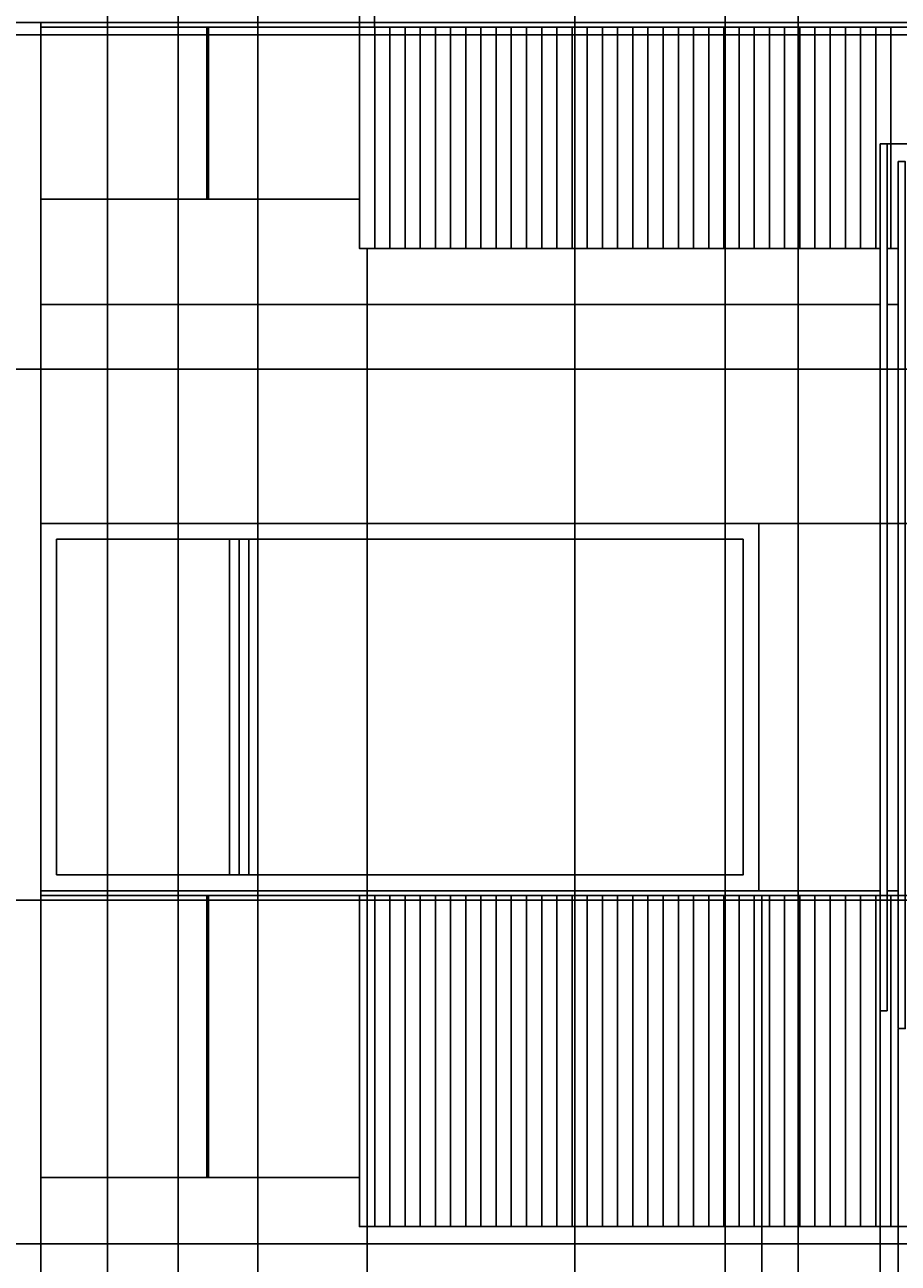
# Model space of a CAD drawing. Units: feet. Extents: x 2193 to 3502, y 890 to 1601.
# Tile 13 of 17: x 3145 to 3281, y 1076 to 1268. Entities that reach past the tile are written whole.
import ezdxf

# ---------------------------------------------------------------- set-up
doc = ezdxf.new("R2010")
doc.units = ezdxf.units.FT
doc.layers.add('A-ANNO-DIMS', color=2, linetype='Continuous', lineweight=18)
doc.layers.add('A-ELEV', color=7, linetype='Continuous', lineweight=25)
doc.styles.get("Standard").update_dxf_attribs({"font": 'arial.ttf'})
doc.dimstyles.get("Standard").update_dxf_attribs({"dimtxt": 0.18, "dimasz": 0.18, "dimexe": 0.18, "dimexo": 0.0625, "dimgap": 0.09, "dimtad": 0, "dimtih": 1, "dimtoh": 1, "dimdec": 0, "dimzin": 0, "dimdsep": 46, "dimlunit": 3, "dimtxsty": 'Standard', "dimcen": 0.09, "dimadec": 0, "dimazin": 0, "dimtfac": 1, "dimtdec": 0, "dimtofl": 0, "dimtmove": 0, "dimatfit": 3, "dimfxl": 1, "dimtolj": 1, "dimtzin": 0, "dimarcsym": 0})

# ---------------------------------------------------------------- blocks, each defined once
blk = doc.blocks.new('*D13')
at = {"layer": 'A-ANNO-DIMS', "color": 0, "lineweight": -2, "transparency": 16777216}
for p, q in [((2934.37, 950.89), (2934.37, 1601.47)), ((2934.55, 1601.29), (3186.64, 1601.29)), ((3439.51, 1601.29), (3187.43, 1601.29)), ((3439.69, 1541.11), (3439.69, 1601.47))]:
    blk.add_line(p, q, dxfattribs=at)
at = {"layer": 'A-ANNO-DIMS', "color": 0, "transparency": 16777216}
for points in [[(2934.55, 1601.32), (2934.55, 1601.26), (2934.37, 1601.29)], [(3439.51, 1601.32), (3439.51, 1601.26), (3439.69, 1601.29)]]:
    blk.add_solid(points, dxfattribs=at)
at = {"layer": 'Defpoints', "color": 0, "transparency": 16777216}
for p in [(3439.69, 1601.29), (3439.69, 1541.04), (2934.37, 950.82)]:
    blk.add_point(p, dxfattribs=at)
at = {"layer": 'A-ANNO-DIMS', "color": 0, "transparency": 16777216, "insert": (3187.03, 1601.29), "char_height": 0.18, "attachment_point": 5}
blk.add_mtext('\\A1;505.3', dxfattribs=at)
blk = doc.blocks.new('*D31')
at = {"layer": 'A-ANNO-DIMS', "color": 0, "lineweight": -2, "transparency": 16777216}
for p, q in [((2760.54, 1541.04), (3501.85, 1541.04)), ((3501.67, 1540.86), (3501.67, 1246.12)), ((3501.67, 951), (3501.67, 1245.75)), ((2762.27, 950.82), (3501.85, 950.82))]:
    blk.add_line(p, q, dxfattribs=at)
at = {"layer": 'A-ANNO-DIMS', "color": 0, "transparency": 16777216}
for points in [[(3501.64, 1540.86), (3501.7, 1540.86), (3501.67, 1541.04)], [(3501.64, 951), (3501.7, 951), (3501.67, 950.82)]]:
    blk.add_solid(points, dxfattribs=at)
at = {"layer": 'Defpoints', "color": 0, "transparency": 16777216}
for p in [(2760.47, 1541.04), (3501.67, 1541.04), (2762.2, 950.82)]:
    blk.add_point(p, dxfattribs=at)
at = {"layer": 'A-ANNO-DIMS', "color": 0, "transparency": 16777216, "insert": (3501.67, 1245.93), "char_height": 0.18, "attachment_point": 5}
blk.add_mtext('\\A1;590.2', dxfattribs=at)
blk = doc.blocks.new('*D61')
at = {"layer": 'A-ANNO-DIMS', "color": 0, "lineweight": -2, "transparency": 16777216}
for p, q in [((2974.12, 1078.97), (2974.12, 890.39)), ((3147.5, 1078.97), (3147.5, 890.39)), ((2974.3, 890.57), (3060.42, 890.57)), ((3147.32, 890.57), (3061.19, 890.57))]:
    blk.add_line(p, q, dxfattribs=at)
at = {"layer": 'A-ANNO-DIMS', "color": 0, "transparency": 16777216}
for points in [[(2974.3, 890.6), (2974.3, 890.54), (2974.12, 890.57)], [(3147.32, 890.6), (3147.32, 890.54), (3147.5, 890.57)]]:
    blk.add_solid(points, dxfattribs=at)
at = {"layer": 'Defpoints', "color": 0, "transparency": 16777216}
for p in [(2974.12, 1079.03), (3147.5, 1079.03), (3147.5, 890.57)]:
    blk.add_point(p, dxfattribs=at)
at = {"layer": 'A-ANNO-DIMS', "color": 0, "transparency": 16777216, "insert": (3060.81, 890.57), "char_height": 0.18, "attachment_point": 5}
blk.add_mtext('\\A1;173.4', dxfattribs=at)
blk = doc.blocks.new('*D62')
at = {"layer": 'A-ANNO-DIMS', "color": 0, "lineweight": -2, "transparency": 16777216}
for p, q in [((2974.18, 1266.71), (3501.85, 1266.71)), ((3501.67, 1266.53), (3501.67, 1173.05)), ((3501.67, 1079.21), (3501.67, 1172.69)), ((2974.18, 1079.03), (3501.85, 1079.03))]:
    blk.add_line(p, q, dxfattribs=at)
at = {"layer": 'A-ANNO-DIMS', "color": 0, "transparency": 16777216}
for points in [[(3501.64, 1266.53), (3501.7, 1266.53), (3501.67, 1266.71)], [(3501.64, 1079.21), (3501.7, 1079.21), (3501.67, 1079.03)]]:
    blk.add_solid(points, dxfattribs=at)
at = {"layer": 'Defpoints', "color": 0, "transparency": 16777216}
for p in [(2974.12, 1266.71), (3501.67, 1266.71), (2974.12, 1079.03)]:
    blk.add_point(p, dxfattribs=at)
at = {"layer": 'A-ANNO-DIMS', "color": 0, "transparency": 16777216, "insert": (3501.67, 1172.87), "char_height": 0.18, "attachment_point": 5}
blk.add_mtext('\\A1;187.68', dxfattribs=at)
blk = doc.blocks.new('*D67')
at = {"layer": 'A-ANNO-DIMS', "color": 0, "lineweight": -2, "transparency": 16777216}
for p, q in [((2980.78, 1214.84), (3501.85, 1214.84)), ((3501.67, 1214.66), (3501.67, 1173.8)), ((3501.67, 1132.57), (3501.67, 1173.43)), ((2980.78, 1132.39), (3501.85, 1132.39))]:
    blk.add_line(p, q, dxfattribs=at)
at = {"layer": 'A-ANNO-DIMS', "color": 0, "transparency": 16777216}
for points in [[(3501.64, 1214.66), (3501.7, 1214.66), (3501.67, 1214.84)], [(3501.64, 1132.57), (3501.7, 1132.57), (3501.67, 1132.39)]]:
    blk.add_solid(points, dxfattribs=at)
at = {"layer": 'Defpoints', "color": 0, "transparency": 16777216}
for p in [(2980.72, 1214.84), (3501.67, 1214.84), (2980.72, 1132.39)]:
    blk.add_point(p, dxfattribs=at)
at = {"layer": 'A-ANNO-DIMS', "color": 0, "transparency": 16777216, "insert": (3501.67, 1173.62), "char_height": 0.18, "attachment_point": 5}
blk.add_mtext('\\A1;82.44', dxfattribs=at)
blk = doc.blocks.new('*D76')
at = {"layer": 'A-ANNO-DIMS', "color": 0, "lineweight": -2, "transparency": 16777216}
for p, q in [((3259.05, 1190.87), (3501.85, 1190.87)), ((3501.67, 1190.69), (3501.67, 1162.17)), ((3501.67, 1133.29), (3501.67, 1161.81)), ((3259.52, 1133.11), (3501.85, 1133.11))]:
    blk.add_line(p, q, dxfattribs=at)
at = {"layer": 'A-ANNO-DIMS', "color": 0, "transparency": 16777216}
for points in [[(3501.64, 1190.69), (3501.7, 1190.69), (3501.67, 1190.87)], [(3501.64, 1133.29), (3501.7, 1133.29), (3501.67, 1133.11)]]:
    blk.add_solid(points, dxfattribs=at)
at = {"layer": 'Defpoints', "color": 0, "transparency": 16777216}
for p in [(3258.98, 1190.87), (3501.67, 1190.87), (3259.46, 1133.11)]:
    blk.add_point(p, dxfattribs=at)
at = {"layer": 'A-ANNO-DIMS', "color": 0, "transparency": 16777216, "insert": (3501.67, 1161.99), "char_height": 0.18, "attachment_point": 5}
blk.add_mtext('\\A1;57.75', dxfattribs=at)
blk = doc.blocks.new('*D80')
at = {"layer": 'A-ANNO-DIMS', "color": 0, "lineweight": -2, "transparency": 16777216}
for p, q in [((3198.15, 1233.5), (3198.15, 890.39)), ((3315.74, 1233.5), (3315.74, 890.39)), ((3198.33, 890.57), (3256.49, 890.57)), ((3315.56, 890.57), (3257.4, 890.57))]:
    blk.add_line(p, q, dxfattribs=at)
at = {"layer": 'A-ANNO-DIMS', "color": 0, "transparency": 16777216}
for points in [[(3198.33, 890.6), (3198.33, 890.54), (3198.15, 890.57)], [(3315.56, 890.6), (3315.56, 890.54), (3315.74, 890.57)]]:
    blk.add_solid(points, dxfattribs=at)
at = {"layer": 'Defpoints', "color": 0, "transparency": 16777216}
for p in [(3198.15, 1233.56), (3315.74, 1233.56), (3315.74, 890.57)]:
    blk.add_point(p, dxfattribs=at)
at = {"layer": 'A-ANNO-DIMS', "color": 0, "transparency": 16777216, "insert": (3256.94, 890.57), "char_height": 0.18, "attachment_point": 5}
blk.add_mtext('\\A1;117.58', dxfattribs=at)
blk = doc.blocks.new('*D83')
at = {"layer": 'A-ANNO-DIMS', "color": 0, "lineweight": -2, "transparency": 16777216}
for p, q in [((3147.5, 1133.05), (3147.5, 890.39)), ((3198.15, 1133.05), (3198.15, 890.39)), ((3147.68, 890.57), (3172.43, 890.57)), ((3197.97, 890.57), (3173.22, 890.57))]:
    blk.add_line(p, q, dxfattribs=at)
at = {"layer": 'A-ANNO-DIMS', "color": 0, "transparency": 16777216}
for points in [[(3147.68, 890.6), (3147.68, 890.54), (3147.5, 890.57)], [(3197.97, 890.6), (3197.97, 890.54), (3198.15, 890.57)]]:
    blk.add_solid(points, dxfattribs=at)
at = {"layer": 'Defpoints', "color": 0, "transparency": 16777216}
for p in [(3147.5, 1133.11), (3198.15, 1133.11), (3198.15, 890.57)]:
    blk.add_point(p, dxfattribs=at)
at = {"layer": 'A-ANNO-DIMS', "color": 0, "transparency": 16777216, "insert": (3172.83, 890.57), "char_height": 0.18, "attachment_point": 5}
blk.add_mtext('\\A1;50.65', dxfattribs=at)
blk = doc.blocks.new('*D84')
at = {"layer": 'A-ANNO-DIMS', "color": 0, "lineweight": -2, "transparency": 16777216}
for p, q in [((3196.98, 1267.98), (3196.98, 1601.47)), ((3197.16, 1601.29), (3197.76, 1601.29)), ((3199.15, 1601.29), (3198.55, 1601.29)), ((3199.33, 1267.98), (3199.33, 1601.47))]:
    blk.add_line(p, q, dxfattribs=at)
at = {"layer": 'A-ANNO-DIMS', "color": 0, "transparency": 16777216}
for points in [[(3197.16, 1601.32), (3197.16, 1601.26), (3196.98, 1601.29)], [(3199.15, 1601.32), (3199.15, 1601.26), (3199.33, 1601.29)]]:
    blk.add_solid(points, dxfattribs=at)
at = {"layer": 'Defpoints', "color": 0, "transparency": 16777216}
for p in [(3199.33, 1601.29), (3196.98, 1267.92), (3199.33, 1267.92)]:
    blk.add_point(p, dxfattribs=at)
at = {"layer": 'A-ANNO-DIMS', "color": 0, "transparency": 16777216, "insert": (3198.15, 1601.29), "char_height": 0.18, "attachment_point": 5}
blk.add_mtext('\\A1;2.358', dxfattribs=at)
blk = doc.blocks.new('*D85')
at = {"layer": 'A-ANNO-DIMS', "color": 0, "lineweight": -2, "transparency": 16777216}
for p, q in [((3259.46, 1133.05), (3259.46, 890.39)), ((3277.81, 1115.17), (3277.81, 890.39)), ((3259.64, 890.57), (3268.25, 890.57)), ((3277.63, 890.57), (3269.02, 890.57))]:
    blk.add_line(p, q, dxfattribs=at)
at = {"layer": 'A-ANNO-DIMS', "color": 0, "transparency": 16777216}
for points in [[(3259.64, 890.6), (3259.64, 890.54), (3259.46, 890.57)], [(3277.63, 890.6), (3277.63, 890.54), (3277.81, 890.57)]]:
    blk.add_solid(points, dxfattribs=at)
at = {"layer": 'Defpoints', "color": 0, "transparency": 16777216}
for p in [(3259.46, 1133.11), (3277.81, 1115.23), (3277.81, 890.57)]:
    blk.add_point(p, dxfattribs=at)
at = {"layer": 'A-ANNO-DIMS', "color": 0, "transparency": 16777216, "insert": (3268.63, 890.57), "char_height": 0.18, "attachment_point": 5}
blk.add_mtext('\\A1;18.35', dxfattribs=at)
blk = doc.blocks.new('*D86')
at = {"layer": 'A-ANNO-DIMS', "color": 0, "lineweight": -2, "transparency": 16777216}
for p, q in [((3277.81, 1115.17), (3277.81, 890.39)), ((3280.64, 1112.39), (3280.64, 890.39)), ((3277.99, 890.57), (3278.83, 890.57)), ((3280.46, 890.57), (3279.62, 890.57))]:
    blk.add_line(p, q, dxfattribs=at)
at = {"layer": 'A-ANNO-DIMS', "color": 0, "transparency": 16777216}
for points in [[(3277.99, 890.6), (3277.99, 890.54), (3277.81, 890.57)], [(3280.46, 890.6), (3280.46, 890.54), (3280.64, 890.57)]]:
    blk.add_solid(points, dxfattribs=at)
at = {"layer": 'Defpoints', "color": 0, "transparency": 16777216}
for p in [(3277.81, 1115.23), (3280.64, 1112.45), (3280.64, 890.57)]:
    blk.add_point(p, dxfattribs=at)
at = {"layer": 'A-ANNO-DIMS', "color": 0, "transparency": 16777216, "insert": (3279.22, 890.57), "char_height": 0.18, "attachment_point": 5}
blk.add_mtext('\\A1;2.832', dxfattribs=at)
blk = doc.blocks.new('*D91')
at = {"layer": 'A-ANNO-DIMS', "color": 0, "lineweight": -2, "transparency": 16777216}
for p, q in [((3277.2, 1267.92), (3501.85, 1267.92)), ((3501.67, 1267.74), (3501.67, 1259.05)), ((3501.67, 1250.01), (3501.67, 1258.69)), ((3277.87, 1249.83), (3501.85, 1249.83))]:
    blk.add_line(p, q, dxfattribs=at)
at = {"layer": 'A-ANNO-DIMS', "color": 0, "transparency": 16777216}
for points in [[(3501.64, 1267.74), (3501.7, 1267.74), (3501.67, 1267.92)], [(3501.64, 1250.01), (3501.7, 1250.01), (3501.67, 1249.83)]]:
    blk.add_solid(points, dxfattribs=at)
at = {"layer": 'Defpoints', "color": 0, "transparency": 16777216}
for p in [(3277.14, 1267.92), (3501.67, 1267.92), (3277.81, 1249.83)]:
    blk.add_point(p, dxfattribs=at)
at = {"layer": 'A-ANNO-DIMS', "color": 0, "transparency": 16777216, "insert": (3501.67, 1258.87), "char_height": 0.18, "attachment_point": 5}
blk.add_mtext('\\A1;18.09', dxfattribs=at)
blk = doc.blocks.new('*D97')
at = {"layer": 'A-ANNO-DIMS', "color": 0, "lineweight": -2, "transparency": 16777216}
for p, q in [((3111.13, 1032.26), (3111.13, 1601.47)), ((3111.31, 1601.29), (3207.6, 1601.29)), ((3304.79, 1601.29), (3208.51, 1601.29)), ((3304.97, 1032.26), (3304.97, 1601.47))]:
    blk.add_line(p, q, dxfattribs=at)
at = {"layer": 'A-ANNO-DIMS', "color": 0, "transparency": 16777216}
for points in [[(3111.31, 1601.32), (3111.31, 1601.26), (3111.13, 1601.29)], [(3304.79, 1601.32), (3304.79, 1601.26), (3304.97, 1601.29)]]:
    blk.add_solid(points, dxfattribs=at)
at = {"layer": 'Defpoints', "color": 0, "transparency": 16777216}
for p in [(3304.97, 1601.29), (3111.13, 1032.19), (3304.97, 1032.19)]:
    blk.add_point(p, dxfattribs=at)
at = {"layer": 'A-ANNO-DIMS', "color": 0, "transparency": 16777216, "insert": (3208.05, 1601.29), "char_height": 0.18, "attachment_point": 5}
blk.add_mtext('\\A1;193.84', dxfattribs=at)
blk = doc.blocks.new('*D100')
at = {"layer": 'A-ANNO-DIMS', "color": 0, "lineweight": -2, "transparency": 16777216}
for p, q in [((3168.83, 1055.37), (3168.83, 1601.47)), ((3169.01, 1601.29), (3216.57, 1601.29)), ((3264.92, 1601.29), (3217.36, 1601.29)), ((3265.1, 1055.37), (3265.1, 1601.47))]:
    blk.add_line(p, q, dxfattribs=at)
at = {"layer": 'A-ANNO-DIMS', "color": 0, "transparency": 16777216}
for points in [[(3169.01, 1601.32), (3169.01, 1601.26), (3168.83, 1601.29)], [(3264.92, 1601.32), (3264.92, 1601.26), (3265.1, 1601.29)]]:
    blk.add_solid(points, dxfattribs=at)
at = {"layer": 'Defpoints', "color": 0, "transparency": 16777216}
for p in [(3265.1, 1601.29), (3168.83, 1055.31), (3265.1, 1055.31)]:
    blk.add_point(p, dxfattribs=at)
at = {"layer": 'A-ANNO-DIMS', "color": 0, "transparency": 16777216, "insert": (3216.97, 1601.29), "char_height": 0.18, "attachment_point": 5}
blk.add_mtext('\\A1;96.27', dxfattribs=at)
blk = doc.blocks.new('*D104')
at = {"layer": 'A-ANNO-DIMS', "color": 0, "lineweight": -2, "transparency": 16777216}
for p, q in [((3157.83, 1001.2), (3157.83, 1601.47)), ((3158.01, 1601.29), (3169.1, 1601.29)), ((3180.99, 1601.29), (3169.89, 1601.29)), ((3181.17, 1001.2), (3181.17, 1601.47))]:
    blk.add_line(p, q, dxfattribs=at)
at = {"layer": 'A-ANNO-DIMS', "color": 0, "transparency": 16777216}
for points in [[(3158.01, 1601.32), (3158.01, 1601.26), (3157.83, 1601.29)], [(3180.99, 1601.32), (3180.99, 1601.26), (3181.17, 1601.29)]]:
    blk.add_solid(points, dxfattribs=at)
at = {"layer": 'Defpoints', "color": 0, "transparency": 16777216}
for p in [(3181.17, 1601.29), (3157.83, 1001.13), (3181.17, 1001.13)]:
    blk.add_point(p, dxfattribs=at)
at = {"layer": 'A-ANNO-DIMS', "color": 0, "transparency": 16777216, "insert": (3169.5, 1601.29), "char_height": 0.18, "attachment_point": 5}
blk.add_mtext('\\A1;23.34', dxfattribs=at)
blk = doc.blocks.new('*D106')
at = {"layer": 'A-ANNO-DIMS', "color": 0, "lineweight": -2, "transparency": 16777216}
for p, q in [((3230.44, 1001.2), (3230.44, 1601.47)), ((3230.62, 1601.29), (3241.72, 1601.29)), ((3253.6, 1601.29), (3242.51, 1601.29)), ((3253.78, 1001.2), (3253.78, 1601.47))]:
    blk.add_line(p, q, dxfattribs=at)
at = {"layer": 'A-ANNO-DIMS', "color": 0, "transparency": 16777216}
for points in [[(3230.62, 1601.32), (3230.62, 1601.26), (3230.44, 1601.29)], [(3253.6, 1601.32), (3253.6, 1601.26), (3253.78, 1601.29)]]:
    blk.add_solid(points, dxfattribs=at)
at = {"layer": 'Defpoints', "color": 0, "transparency": 16777216}
for p in [(3253.78, 1601.29), (3230.44, 1001.13), (3253.78, 1001.13)]:
    blk.add_point(p, dxfattribs=at)
at = {"layer": 'A-ANNO-DIMS', "color": 0, "transparency": 16777216, "insert": (3242.11, 1601.29), "char_height": 0.18, "attachment_point": 5}
blk.add_mtext('\\A1;23.34', dxfattribs=at)

msp = doc.modelspace()

# ---------------------------------------------------------------- linework, layer by layer
at = {"layer": 'A-ELEV'}
for p, q in [((3147.5022, 1241.1967), (3196.9758, 1241.1967)), ((3147.5022, 1224.865), (3277.8077, 1224.865)), ((3278.9051, 1224.865), (3280.6398, 1224.865)), ((3147.5022, 1089.3627), (3196.9758, 1089.3627))]:
    msp.add_line(p, q, dxfattribs=at)
for points in [[(2974.116, 1266.7092), (3147.5022, 1266.7092), (3147.5022, 1268.6599), (2974.116, 1268.6599)], [(2974.116, 1079.031), (3147.5022, 1079.031), (3147.5022, 1266.7092), (2974.116, 1266.7092)], [(3277.8077, 1249.8256), (3278.9051, 1249.8256), (3278.9051, 1115.2331), (3277.8077, 1115.2331)], [(3280.6398, 1247.0422), (3281.7371, 1247.0422), (3281.7371, 1112.4498), (3280.6398, 1112.4498)], [(3147.5022, 1133.8558), (3258.9838, 1133.8558), (3258.9838, 1190.8659), (3147.5022, 1190.8659)], [(3149.9473, 1136.3009), (3256.5386, 1136.3009), (3256.5386, 1188.4208), (3149.9473, 1188.4208)], [(3176.7885, 1188.4208), (3178.3021, 1188.4208), (3178.3021, 1136.3009), (3176.7885, 1136.3009)], [(3178.3021, 1188.4208), (3179.8157, 1188.4208), (3179.8157, 1136.3009), (3178.3021, 1136.3009)], [(3173.2631, 1133.1128), (3173.5128, 1133.1128), (3173.5128, 1089.3627), (3173.2631, 1089.3627)]]:
    msp.add_lwpolyline(points, close=True, dxfattribs=at)
for points in [[(3378.849, 1267.9169), (3147.5022, 1267.9169), (3147.5022, 1268.6599), (3378.849, 1268.6599)], [(3173.5128, 1267.9169), (3173.5128, 1241.1967), (3173.2631, 1241.1967), (3173.2631, 1267.9169)], [(3277.8077, 1233.561), (3196.9758, 1233.561), (3196.9758, 1267.9169)], [(3199.3336, 1267.9169), (3199.3336, 1233.561), (3198.1547, 1233.561)], [(3201.6915, 1267.9169), (3201.6915, 1233.561), (3200.5126, 1233.561)], [(3204.0493, 1267.9169), (3204.0493, 1233.561), (3202.8704, 1233.561)], [(3206.4072, 1267.9169), (3206.4072, 1233.561), (3205.2282, 1233.561)], [(3208.765, 1267.9169), (3208.765, 1233.561), (3207.5861, 1233.561)], [(3211.1228, 1267.9169), (3211.1228, 1233.561), (3209.9439, 1233.561)], [(3213.4807, 1267.9169), (3213.4807, 1233.561), (3212.3017, 1233.561)], [(3215.8385, 1267.9169), (3215.8385, 1233.561), (3214.6596, 1233.561)], [(3218.1963, 1267.9169), (3218.1963, 1233.561), (3217.0174, 1233.561)], [(3220.5542, 1267.9169), (3220.5542, 1233.561), (3219.3753, 1233.561)], [(3222.912, 1267.9169), (3222.912, 1233.561), (3221.7331, 1233.561)], [(3225.2698, 1267.9169), (3225.2698, 1233.561), (3224.0909, 1233.561)], [(3227.6277, 1267.9169), (3227.6277, 1233.561), (3226.4488, 1233.561)], [(3229.9855, 1267.9169), (3229.9855, 1233.561), (3228.8066, 1233.561)], [(3232.3434, 1267.9169), (3232.3434, 1233.561), (3231.1644, 1233.561)], [(3234.7012, 1267.9169), (3234.7012, 1233.561), (3233.5223, 1233.561)], [(3237.059, 1267.9169), (3237.059, 1233.561), (3235.8801, 1233.561)], [(3239.4169, 1267.9169), (3239.4169, 1233.561), (3238.238, 1233.561)], [(3241.7747, 1267.9169), (3241.7747, 1233.561), (3240.5958, 1233.561)], [(3244.1325, 1267.9169), (3244.1325, 1233.561), (3242.9536, 1233.561)], [(3246.4904, 1267.9169), (3246.4904, 1233.561), (3245.3115, 1233.561)], [(3248.8482, 1267.9169), (3248.8482, 1233.561), (3247.6693, 1233.561)], [(3251.2061, 1267.9169), (3251.2061, 1233.561), (3250.0271, 1233.561)], [(3253.5639, 1267.9169), (3253.5639, 1233.561), (3252.385, 1233.561)], [(3255.9217, 1267.9169), (3255.9217, 1233.561), (3254.7428, 1233.561)], [(3258.2796, 1267.9169), (3258.2796, 1233.561), (3257.1006, 1233.561)], [(3260.6374, 1267.9169), (3260.6374, 1233.561), (3259.4585, 1233.561)], [(3262.9952, 1267.9169), (3262.9952, 1233.561), (3261.8163, 1233.561)], [(3265.3531, 1267.9169), (3265.3531, 1233.561), (3264.1742, 1233.561)], [(3267.7109, 1267.9169), (3267.7109, 1233.561), (3266.532, 1233.561)], [(3270.0688, 1267.9169), (3270.0688, 1233.561), (3268.8898, 1233.561)], [(3272.4266, 1267.9169), (3272.4266, 1233.561), (3271.2477, 1233.561)], [(3274.7844, 1267.9169), (3274.7844, 1233.561), (3273.6055, 1233.561)], [(3277.1423, 1267.9169), (3277.1423, 1233.561), (3275.9633, 1233.561)], [(3279.5001, 1267.9169), (3279.5001, 1233.561), (3278.9051, 1233.561)], [(3280.6398, 1233.561), (3278.9051, 1233.561)], [(3277.8077, 1133.1128), (3147.5022, 1133.1128), (3147.5022, 1133.8558), (3277.8077, 1133.8558)], [(3277.8077, 1133.8558), (3147.5022, 1133.8558), (3147.5022, 1089.3627)], [(3315.7352, 1133.1128), (3315.7352, 1081.7269), (3196.9758, 1081.7269), (3196.9758, 1133.1128)], [(3198.1547, 1133.1128), (3199.3336, 1133.1128), (3199.3336, 1081.7269), (3198.1547, 1081.7269)], [(3200.5126, 1133.1128), (3201.6915, 1133.1128), (3201.6915, 1081.7269), (3200.5126, 1081.7269)], [(3202.8704, 1133.1128), (3204.0493, 1133.1128), (3204.0493, 1081.7269), (3202.8704, 1081.7269)], [(3205.2282, 1133.1128), (3206.4072, 1133.1128), (3206.4072, 1081.7269), (3205.2282, 1081.7269)], [(3207.5861, 1133.1128), (3208.765, 1133.1128), (3208.765, 1081.7269), (3207.5861, 1081.7269)], [(3209.9439, 1133.1128), (3211.1228, 1133.1128), (3211.1228, 1081.7269), (3209.9439, 1081.7269)], [(3212.3017, 1133.1128), (3213.4807, 1133.1128), (3213.4807, 1081.7269), (3212.3017, 1081.7269)], [(3214.6596, 1133.1128), (3215.8385, 1133.1128), (3215.8385, 1081.7269), (3214.6596, 1081.7269)], [(3217.0174, 1133.1128), (3218.1963, 1133.1128), (3218.1963, 1081.7269), (3217.0174, 1081.7269)], [(3219.3753, 1133.1128), (3220.5542, 1133.1128), (3220.5542, 1081.7269), (3219.3753, 1081.7269)], [(3221.7331, 1133.1128), (3222.912, 1133.1128), (3222.912, 1081.7269), (3221.7331, 1081.7269)], [(3224.0909, 1133.1128), (3225.2698, 1133.1128), (3225.2698, 1081.7269), (3224.0909, 1081.7269)], [(3226.4488, 1133.1128), (3227.6277, 1133.1128), (3227.6277, 1081.7269), (3226.4488, 1081.7269)], [(3228.8066, 1133.1128), (3229.9855, 1133.1128), (3229.9855, 1081.7269), (3228.8066, 1081.7269)], [(3231.1644, 1133.1128), (3232.3434, 1133.1128), (3232.3434, 1081.7269), (3231.1644, 1081.7269)], [(3233.5223, 1133.1128), (3234.7012, 1133.1128), (3234.7012, 1081.7269), (3233.5223, 1081.7269)], [(3235.8801, 1133.1128), (3237.059, 1133.1128), (3237.059, 1081.7269), (3235.8801, 1081.7269)], [(3238.238, 1133.1128), (3239.4169, 1133.1128), (3239.4169, 1081.7269), (3238.238, 1081.7269)], [(3240.5958, 1133.1128), (3241.7747, 1133.1128), (3241.7747, 1081.7269), (3240.5958, 1081.7269)], [(3242.9536, 1133.1128), (3244.1325, 1133.1128), (3244.1325, 1081.7269), (3242.9536, 1081.7269)], [(3245.3115, 1133.1128), (3246.4904, 1133.1128), (3246.4904, 1081.7269), (3245.3115, 1081.7269)], [(3247.6693, 1133.1128), (3248.8482, 1133.1128), (3248.8482, 1081.7269), (3247.6693, 1081.7269)], [(3250.0271, 1133.1128), (3251.2061, 1133.1128), (3251.2061, 1081.7269), (3250.0271, 1081.7269)], [(3252.385, 1133.1128), (3253.5639, 1133.1128), (3253.5639, 1081.7269), (3252.385, 1081.7269)], [(3254.7428, 1133.1128), (3255.9217, 1133.1128), (3255.9217, 1081.7269), (3254.7428, 1081.7269)], [(3257.1006, 1133.1128), (3258.2796, 1133.1128), (3258.2796, 1081.7269), (3257.1006, 1081.7269)], [(3259.4585, 1133.1128), (3260.6374, 1133.1128), (3260.6374, 1081.7269), (3259.4585, 1081.7269)], [(3261.8163, 1133.1128), (3262.9952, 1133.1128), (3262.9952, 1081.7269), (3261.8163, 1081.7269)], [(3264.1742, 1133.1128), (3265.3531, 1133.1128), (3265.3531, 1081.7269), (3264.1742, 1081.7269)], [(3266.532, 1133.1128), (3267.7109, 1133.1128), (3267.7109, 1081.7269), (3266.532, 1081.7269)], [(3268.8898, 1133.1128), (3270.0688, 1133.1128), (3270.0688, 1081.7269), (3268.8898, 1081.7269)], [(3271.2477, 1133.1128), (3272.4266, 1133.1128), (3272.4266, 1081.7269), (3271.2477, 1081.7269)], [(3273.6055, 1133.1128), (3274.7844, 1133.1128), (3274.7844, 1081.7269), (3273.6055, 1081.7269)], [(3275.9633, 1133.1128), (3277.1423, 1133.1128), (3277.1423, 1081.7269), (3275.9633, 1081.7269)], [(3278.9051, 1133.1128), (3279.5001, 1133.1128), (3279.5001, 1081.7269), (3278.3212, 1081.7269)], [(3278.9051, 1133.8558), (3280.6398, 1133.8558)], [(3280.6398, 1133.8558), (3278.9051, 1133.8558)], [(3280.6398, 1133.1128), (3278.9051, 1133.1128)]]:
    msp.add_lwpolyline(points, dxfattribs=at)

# ---------------------------------------------------------------- dimensions: what is measured, and where the dimension line sits
at = {"layer": 'A-ANNO-DIMS'}
for base, p1, p2, override, picture, middle in [((3439.6901, 1601.2941), (2934.3742, 950.8228), (3439.6901, 1541.0441), {"dimdec": 1, "dimlfac": 1, "dimrnd": 0, "dimzin": 0, "dimdsep": 46, "dimlunit": 2}, '*D13', (3187.0321, 1601.2941)), ((3304.9731, 1601.2941), (3111.1302, 1032.1935), (3304.9731, 1032.1935), {"dimdec": 2, "dimlfac": 1, "dimrnd": 0, "dimzin": 0, "dimdsep": 46, "dimlunit": 2}, '*D97', (3208.0516, 1601.2941)), ((3181.1661, 1601.2941), (3157.8263, 1001.1334), (3181.1661, 1001.1334), {"dimdec": 2, "dimlfac": 1, "dimrnd": 0, "dimzin": 0, "dimdsep": 46, "dimlunit": 2}, '*D104', (3169.4962, 1601.2941)), ((3265.1012, 1601.2941), (3168.8336, 1055.3069), (3265.1012, 1055.3069), {"dimdec": 2, "dimlfac": 1, "dimrnd": 0, "dimzin": 0, "dimdsep": 46, "dimlunit": 2}, '*D100', (3216.9674, 1601.2941)), ((3199.3336, 1601.2941), (3196.9758, 1267.9169), (3199.3336, 1267.9169), {"dimdec": 3, "dimlfac": 1, "dimrnd": 0, "dimzin": 0, "dimdsep": 46, "dimlunit": 2}, '*D84', (3198.1547, 1601.2941)), ((3253.781, 1601.2941), (3230.4412, 1001.1334), (3253.781, 1001.1334), {"dimdec": 2, "dimlfac": 1, "dimrnd": 0, "dimzin": 0, "dimdsep": 46, "dimlunit": 2}, '*D106', (3242.1111, 1601.2941)), ((3315.7352, 890.5728), (3198.1547, 1233.561), (3315.7352, 1233.561), {"dimdec": 2, "dimlfac": 1, "dimrnd": 0, "dimzin": 0, "dimdsep": 46, "dimlunit": 2}, '*D80', (3256.9449, 890.5728)), ((3198.1547, 890.5728), (3147.5022, 1133.1128), (3198.1547, 1133.1128), {"dimdec": 2, "dimlfac": 1, "dimrnd": 0, "dimzin": 0, "dimdsep": 46, "dimlunit": 2}, '*D83', (3172.8284, 890.5728)), ((3277.8077, 890.5728), (3259.4585, 1133.1128), (3277.8077, 1115.2331), {"dimdec": 2, "dimlfac": 1, "dimrnd": 0, "dimzin": 0, "dimdsep": 46, "dimlunit": 2}, '*D85', (3268.6331, 890.5728)), ((3280.6398, 890.5728), (3277.8077, 1115.2331), (3280.6398, 1112.4498), {"dimdec": 3, "dimlfac": 1, "dimrnd": 0, "dimzin": 0, "dimdsep": 46, "dimlunit": 2}, '*D86', (3279.2237, 890.5728)), ((3147.5022, 890.5728), (2974.116, 1079.031), (3147.5022, 1079.031), {"dimdec": 1, "dimlfac": 1, "dimrnd": 0, "dimzin": 0, "dimdsep": 46, "dimlunit": 2}, '*D61', (3060.8091, 890.5728))]:
    dim = msp.add_linear_dim(base=base, p1=p1, p2=p2, dimstyle='Standard', override=override, dxfattribs=at)
    dim.commit()
    dim.dimension.update_dxf_attribs({"geometry": picture, "text_midpoint": middle})
for base, p1, p2, override, picture, middle in [((3501.6716, 1541.0441), (2762.2048, 950.8228), (2760.4733, 1541.0441), {"dimdec": 1, "dimlfac": 1, "dimrnd": 0, "dimzin": 0, "dimdsep": 46, "dimlunit": 2}, '*D31', (3501.6716, 1245.9334)), ((3501.6716, 1267.9169), (3277.8077, 1249.8256), (3277.1423, 1267.9169), {"dimdec": 2, "dimlfac": 1, "dimrnd": 0, "dimzin": 0, "dimdsep": 46, "dimlunit": 2}, '*D91', (3501.6716, 1258.8712)), ((3501.6716, 1266.7092), (2974.116, 1079.031), (2974.116, 1266.7092), {"dimdec": 2, "dimlfac": 1, "dimrnd": 0, "dimzin": 0, "dimdsep": 46, "dimlunit": 2}, '*D62', (3501.6716, 1172.8701)), ((3501.6716, 1214.8367), (2980.7151, 1132.3937), (2980.7151, 1214.8367), {"dimdec": 2, "dimlfac": 1, "dimrnd": 0, "dimzin": 0, "dimdsep": 46, "dimlunit": 2}, '*D67', (3501.6716, 1173.6152)), ((3501.6716, 1190.8659), (3259.4585, 1133.1128), (3258.9838, 1190.8659), {"dimdec": 2, "dimlfac": 1, "dimrnd": 0, "dimzin": 0, "dimdsep": 46, "dimlunit": 2}, '*D76', (3501.6716, 1161.9893))]:
    dim = msp.add_linear_dim(base=base, p1=p1, p2=p2, angle=90, dimstyle='Standard', override=override, dxfattribs=at)
    dim.commit()
    dim.dimension.update_dxf_attribs({"geometry": picture, "text_midpoint": middle})

doc.saveas('drawing.dxf')
